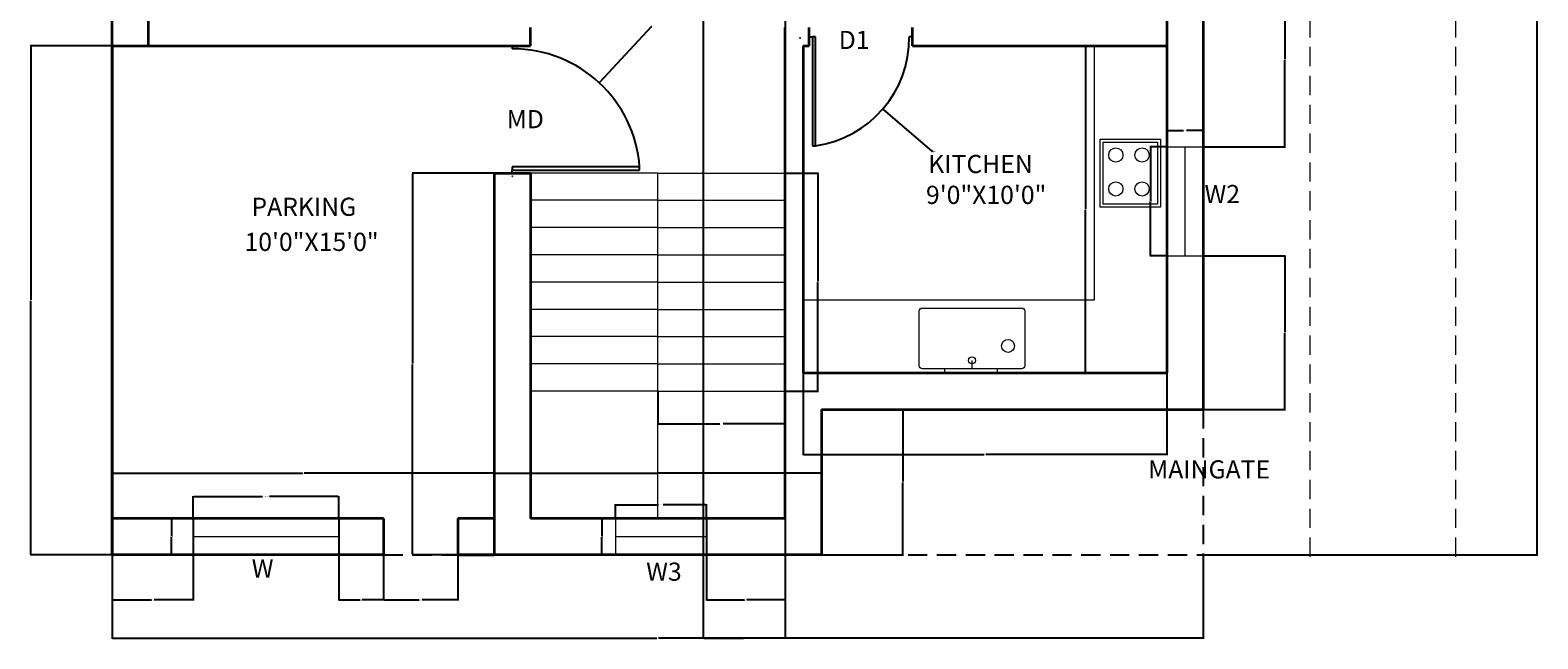
# Model space of a CAD drawing. Units: inches. Extents: x 2906 to 3403, y 1614 to 2150.
# Tile 1 of 4: x 2906 to 3403, y 1614 to 1814. Entities that reach past the tile are written whole.
import ezdxf

# ---------------------------------------------------------------- set-up
doc = ezdxf.new("R2010")
doc.units = ezdxf.units.IN
doc.linetypes.add('DASHED2', pattern=[9.525, 6.35, -3.175])
for name, color, linetype, lineweight in [('A-ANNO-DIMS', 2, 'Continuous', 18), ('A-ANNO-TEXT', 220, 'Continuous', 18), ('A-AREA-IDEN', 220, 'Continuous', 25), ('A-DOOR', 40, 'Continuous', 25), ('A-EQPM', 121, 'Continuous', 18), ('A-FLOR-CASE', 121, 'Continuous', 18), ('A-FLOR-FIXT', 121, 'Continuous', 18), ('A-FLOR-STRS', 191, 'Continuous', 18), ('A-GLAZ', 2, 'Continuous', 18), ('A-WALL', 191, 'Continuous', 35), ('C-PROP', 255, 'DASHED2', 25), ('C-ROAD', 255, 'DASHED2', 18)]:
    doc.layers.add(name, color=color, linetype=linetype, lineweight=lineweight)
doc.styles.get("Standard").update_dxf_attribs({"font": 'arial.ttf'})
doc.dimstyles.get("Standard").update_dxf_attribs({"dimtxt": 0.18, "dimasz": 0.18, "dimexe": 0.18, "dimexo": 0.0625, "dimgap": 0.09, "dimtad": 0, "dimtih": 1, "dimtoh": 1, "dimdec": 4, "dimzin": 0, "dimdsep": 46, "dimtxsty": 'Standard', "dimcen": 0.09, "dimadec": 0, "dimazin": 0, "dimtfac": 1, "dimtdec": 4, "dimtofl": 0, "dimtmove": 0, "dimatfit": 3, "dimfxl": 1, "dimtolj": 1, "dimtzin": 0, "dimarcsym": 0})

# ---------------------------------------------------------------- blocks, each defined once
blk = doc.blocks.new('WINDOW-48')
for p, q in [((0, 12), (0, 0)), ((48, 12), (48, 0)), ((0, 6), (48, 6))]:
    blk.add_line(p, q)
blk = doc.blocks.new('WINDOW-36')
for p, q in [((12, 36), (0, 36)), ((6, 36), (6, 0)), ((12, 0), (0, 0))]:
    blk.add_line(p, q)
blk = doc.blocks.new('WINDOW-30')
for p, q in [((0, 12), (0, 0)), ((30, 12), (30, 0)), ((0, 6), (30, 6))]:
    blk.add_line(p, q)
blk = doc.blocks.new('STAIR-FLIGHT-42')
for p, q in [((0, 72), (42, 72)), ((0, 63), (42, 63)), ((0, 54), (42, 54)), ((0, 45), (42, 45)), ((0, 36), (42, 36)), ((0, 27), (42, 27)), ((0, 18), (42, 18)), ((0, 9), (42, 9)), ((0, 0), (42, 0))]:
    blk.add_line(p, q)
blk = doc.blocks.new('*D18')
at = {"layer": 'A-ANNO-DIMS', "color": 0, "lineweight": -2, "transparency": 16777216}
for p, q in [((2959.37, 1653.32), (2959.37, 1660.63)), ((2959.55, 1660.45), (2982.25, 1660.45)), ((3007.19, 1660.45), (2984.49, 1660.45)), ((3007.37, 1653.32), (3007.37, 1660.63))]:
    blk.add_line(p, q, dxfattribs=at)
at = {"layer": 'A-ANNO-DIMS', "color": 0, "transparency": 16777216}
for points in [[(2959.55, 1660.48), (2959.55, 1660.42), (2959.37, 1660.45)], [(3007.19, 1660.48), (3007.19, 1660.42), (3007.37, 1660.45)]]:
    blk.add_solid(points, dxfattribs=at)
at = {"layer": 'Defpoints', "color": 0, "transparency": 16777216}
for p in [(3007.37, 1660.45), (2959.37, 1653.25), (3007.37, 1653.25)]:
    blk.add_point(p, dxfattribs=at)
at = {"layer": 'A-ANNO-DIMS', "color": 0, "transparency": 16777216, "insert": (2983.37, 1660.45), "char_height": 0.18, "attachment_point": 5}
blk.add_mtext('\\A1;WINDOW 48 TYP.', dxfattribs=at)
blk = doc.blocks.new('*D19')
at = {"layer": 'A-ANNO-DIMS', "color": 0, "lineweight": -2, "transparency": 16777216}
for p, q in [((2959.31, 1653.25), (2951.99, 1653.25)), ((2952.17, 1653.07), (2952.17, 1647.43)), ((2952.17, 1641.43), (2952.17, 1647.07)), ((2959.31, 1641.25), (2951.99, 1641.25))]:
    blk.add_line(p, q, dxfattribs=at)
at = {"layer": 'A-ANNO-DIMS', "color": 0, "transparency": 16777216}
for points in [[(2952.14, 1653.07), (2952.2, 1653.07), (2952.17, 1653.25)], [(2952.14, 1641.43), (2952.2, 1641.43), (2952.17, 1641.25)]]:
    blk.add_solid(points, dxfattribs=at)
at = {"layer": 'Defpoints', "color": 0, "transparency": 16777216}
for p in [(2952.17, 1653.25), (2959.37, 1653.25), (2959.37, 1641.25)]:
    blk.add_point(p, dxfattribs=at)
at = {"layer": 'A-ANNO-DIMS', "color": 0, "transparency": 16777216, "insert": (2952.17, 1647.25), "char_height": 0.18, "attachment_point": 5}
blk.add_mtext('\\A1;12 TYP.', dxfattribs=at)
blk = doc.blocks.new('*D22')
at = {"layer": 'A-ANNO-DIMS', "color": 0, "lineweight": -2, "transparency": 16777216}
for p, q in [((3280.57, 1775.89), (3275.05, 1775.89)), ((3275.23, 1775.71), (3275.23, 1758.08)), ((3275.23, 1740.07), (3275.23, 1757.71)), ((3280.57, 1739.89), (3275.05, 1739.89))]:
    blk.add_line(p, q, dxfattribs=at)
at = {"layer": 'A-ANNO-DIMS', "color": 0, "transparency": 16777216}
for points in [[(3275.2, 1775.71), (3275.26, 1775.71), (3275.23, 1775.89)], [(3275.2, 1740.07), (3275.26, 1740.07), (3275.23, 1739.89)]]:
    blk.add_solid(points, dxfattribs=at)
at = {"layer": 'Defpoints', "color": 0, "transparency": 16777216}
for p in [(3280.63, 1775.89), (3275.23, 1739.89), (3280.63, 1739.89)]:
    blk.add_point(p, dxfattribs=at)
at = {"layer": 'A-ANNO-DIMS', "color": 0, "transparency": 16777216, "insert": (3275.23, 1757.89), "char_height": 0.18, "attachment_point": 5}
blk.add_mtext('\\A1;W2 36 TYP.', dxfattribs=at)
blk = doc.blocks.new('*D23')
at = {"layer": 'A-ANNO-DIMS', "color": 0, "lineweight": -2, "transparency": 16777216}
for p, q in [((3280.63, 1775.96), (3280.63, 1781.47)), ((3280.81, 1781.29), (3286.11, 1781.29)), ((3292.45, 1781.29), (3287.15, 1781.29)), ((3292.63, 1775.96), (3292.63, 1781.47))]:
    blk.add_line(p, q, dxfattribs=at)
at = {"layer": 'A-ANNO-DIMS', "color": 0, "transparency": 16777216}
for points in [[(3280.81, 1781.32), (3280.81, 1781.26), (3280.63, 1781.29)], [(3292.45, 1781.32), (3292.45, 1781.26), (3292.63, 1781.29)]]:
    blk.add_solid(points, dxfattribs=at)
at = {"layer": 'Defpoints', "color": 0, "transparency": 16777216}
for p in [(3280.63, 1781.29), (3280.63, 1775.89), (3292.63, 1775.89)]:
    blk.add_point(p, dxfattribs=at)
at = {"layer": 'A-ANNO-DIMS', "color": 0, "transparency": 16777216, "insert": (3286.63, 1781.29), "char_height": 0.18, "attachment_point": 5}
blk.add_mtext('\\A1;12 TYP.', dxfattribs=at)
blk = doc.blocks.new('*D24')
at = {"layer": 'A-ANNO-DIMS', "color": 0, "lineweight": -2, "transparency": 16777216}
for p, q in [((3098.66, 1653.32), (3098.66, 1657.93)), ((3098.84, 1657.75), (3112.91, 1657.75)), ((3128.48, 1657.75), (3114.42, 1657.75)), ((3128.66, 1653.32), (3128.66, 1657.93))]:
    blk.add_line(p, q, dxfattribs=at)
at = {"layer": 'A-ANNO-DIMS', "color": 0, "transparency": 16777216}
for points in [[(3098.84, 1657.78), (3098.84, 1657.72), (3098.66, 1657.75)], [(3128.48, 1657.78), (3128.48, 1657.72), (3128.66, 1657.75)]]:
    blk.add_solid(points, dxfattribs=at)
at = {"layer": 'Defpoints', "color": 0, "transparency": 16777216}
for p in [(3128.66, 1657.75), (3098.66, 1653.25), (3128.66, 1653.25)]:
    blk.add_point(p, dxfattribs=at)
at = {"layer": 'A-ANNO-DIMS', "color": 0, "transparency": 16777216, "insert": (3113.66, 1657.75), "char_height": 0.18, "attachment_point": 5}
blk.add_mtext('\\A1;W3 30 TYP.', dxfattribs=at)
blk = doc.blocks.new('*D25')
at = {"layer": 'A-ANNO-DIMS', "color": 0, "lineweight": -2, "transparency": 16777216}
for p, q in [((3098.6, 1653.25), (3093.98, 1653.25)), ((3094.16, 1653.07), (3094.16, 1647.43)), ((3094.16, 1641.43), (3094.16, 1647.07)), ((3098.6, 1641.25), (3093.98, 1641.25))]:
    blk.add_line(p, q, dxfattribs=at)
at = {"layer": 'A-ANNO-DIMS', "color": 0, "transparency": 16777216}
for points in [[(3094.13, 1653.07), (3094.19, 1653.07), (3094.16, 1653.25)], [(3094.13, 1641.43), (3094.19, 1641.43), (3094.16, 1641.25)]]:
    blk.add_solid(points, dxfattribs=at)
at = {"layer": 'Defpoints', "color": 0, "transparency": 16777216}
for p in [(3094.16, 1653.25), (3098.66, 1653.25), (3098.66, 1641.25)]:
    blk.add_point(p, dxfattribs=at)
at = {"layer": 'A-ANNO-DIMS', "color": 0, "transparency": 16777216, "insert": (3094.16, 1647.25), "char_height": 0.18, "attachment_point": 5}
blk.add_mtext('\\A1;12 TYP.', dxfattribs=at)
blk = doc.blocks.new('*D32')
at = {"layer": 'A-ANNO-DIMS', "color": 0, "lineweight": -2, "transparency": 16777216}
for p, q in [((3154.7, 1767.25), (3165.61, 1767.25)), ((3165.43, 1767.07), (3165.43, 1731.44)), ((3165.43, 1695.43), (3165.43, 1731.07)), ((3154.7, 1695.25), (3165.61, 1695.25))]:
    blk.add_line(p, q, dxfattribs=at)
at = {"layer": 'A-ANNO-DIMS', "color": 0, "transparency": 16777216}
for points in [[(3165.4, 1767.07), (3165.46, 1767.07), (3165.43, 1767.25)], [(3165.4, 1695.43), (3165.46, 1695.43), (3165.43, 1695.25)]]:
    blk.add_solid(points, dxfattribs=at)
at = {"layer": 'Defpoints', "color": 0, "transparency": 16777216}
for p in [(3154.63, 1767.25), (3165.43, 1767.25), (3154.63, 1695.25)]:
    blk.add_point(p, dxfattribs=at)
at = {"layer": 'A-ANNO-DIMS', "color": 0, "transparency": 16777216, "insert": (3165.43, 1731.25), "char_height": 0.18, "attachment_point": 5}
blk.add_mtext('\\A1;FLIGHT 72 TYP.', dxfattribs=at)
blk = doc.blocks.new('*D33')
at = {"layer": 'A-ANNO-DIMS', "color": 0, "lineweight": -2, "transparency": 16777216}
for p, q in [((3112.63, 1695.19), (3112.63, 1684.27)), ((3154.63, 1695.19), (3154.63, 1684.27)), ((3112.81, 1684.45), (3133.1, 1684.45)), ((3154.45, 1684.45), (3134.16, 1684.45))]:
    blk.add_line(p, q, dxfattribs=at)
at = {"layer": 'A-ANNO-DIMS', "color": 0, "transparency": 16777216}
for points in [[(3112.81, 1684.48), (3112.81, 1684.42), (3112.63, 1684.45)], [(3154.45, 1684.48), (3154.45, 1684.42), (3154.63, 1684.45)]]:
    blk.add_solid(points, dxfattribs=at)
at = {"layer": 'Defpoints', "color": 0, "transparency": 16777216}
for p in [(3112.63, 1695.25), (3154.63, 1695.25), (3154.63, 1684.45)]:
    blk.add_point(p, dxfattribs=at)
at = {"layer": 'A-ANNO-DIMS', "color": 0, "transparency": 16777216, "insert": (3133.63, 1684.45), "char_height": 0.18, "attachment_point": 5}
blk.add_mtext('\\A1;42 TYP.', dxfattribs=at)
blk = doc.blocks.new('*D40')
at = {"layer": 'A-ANNO-DIMS', "color": 0, "lineweight": -2, "transparency": 16777216}
for p, q in [((2932.63, 1641.19), (2932.63, 1613.51)), ((3292.63, 1641.19), (3292.63, 1613.51)), ((2932.81, 1613.69), (3112.34, 1613.69)), ((3292.45, 1613.69), (3112.92, 1613.69))]:
    blk.add_line(p, q, dxfattribs=at)
at = {"layer": 'A-ANNO-DIMS', "color": 0, "transparency": 16777216}
for points in [[(2932.81, 1613.72), (2932.81, 1613.66), (2932.63, 1613.69)], [(3292.45, 1613.72), (3292.45, 1613.66), (3292.63, 1613.69)]]:
    blk.add_solid(points, dxfattribs=at)
at = {"layer": 'Defpoints', "color": 0, "transparency": 16777216}
for p in [(2932.63, 1641.25), (3292.63, 1641.25), (3292.63, 1613.69)]:
    blk.add_point(p, dxfattribs=at)
at = {"layer": 'A-ANNO-DIMS', "color": 0, "transparency": 16777216, "insert": (3112.63, 1613.69), "char_height": 0.18, "attachment_point": 5}
blk.add_mtext('\\A1;360', dxfattribs=at)
blk = doc.blocks.new('*D41')
at = {"layer": 'A-ANNO-DIMS', "color": 0, "lineweight": -2, "transparency": 16777216}
for p, q in [((3292.7, 2121.25), (3403.01, 2121.25)), ((3402.83, 2121.07), (3402.83, 1881.44)), ((3402.83, 1641.43), (3402.83, 1881.07)), ((3292.7, 1641.25), (3403.01, 1641.25))]:
    blk.add_line(p, q, dxfattribs=at)
at = {"layer": 'A-ANNO-DIMS', "color": 0, "transparency": 16777216}
for points in [[(3402.8, 2121.07), (3402.86, 2121.07), (3402.83, 2121.25)], [(3402.8, 1641.43), (3402.86, 1641.43), (3402.83, 1641.25)]]:
    blk.add_solid(points, dxfattribs=at)
at = {"layer": 'Defpoints', "color": 0, "transparency": 16777216}
for p in [(3292.63, 2121.25), (3402.83, 2121.25), (3292.63, 1641.25)]:
    blk.add_point(p, dxfattribs=at)
at = {"layer": 'A-ANNO-DIMS', "color": 0, "transparency": 16777216, "insert": (3402.83, 1881.25), "char_height": 0.18, "attachment_point": 5}
blk.add_mtext('\\A1;480', dxfattribs=at)
blk = doc.blocks.new('*D48')
at = {"layer": 'A-ANNO-DIMS', "color": 0, "lineweight": -2, "transparency": 16777216}
for p, q in [((2932.57, 1809.25), (2905.55, 1809.25)), ((2905.73, 1809.07), (2905.73, 1725.44)), ((2905.73, 1641.43), (2905.73, 1725.07)), ((2932.57, 1641.25), (2905.55, 1641.25))]:
    blk.add_line(p, q, dxfattribs=at)
at = {"layer": 'A-ANNO-DIMS', "color": 0, "transparency": 16777216}
for points in [[(2905.7, 1809.07), (2905.76, 1809.07), (2905.73, 1809.25)], [(2905.7, 1641.43), (2905.76, 1641.43), (2905.73, 1641.25)]]:
    blk.add_solid(points, dxfattribs=at)
at = {"layer": 'Defpoints', "color": 0, "transparency": 16777216}
for p in [(2905.73, 1809.25), (2932.63, 1809.25), (2932.63, 1641.25)]:
    blk.add_point(p, dxfattribs=at)
at = {"layer": 'A-ANNO-DIMS', "color": 0, "transparency": 16777216, "insert": (2905.73, 1725.25), "char_height": 0.18, "attachment_point": 5}
blk.add_mtext('\\A1;168', dxfattribs=at)
blk = doc.blocks.new('*D52')
at = {"layer": 'A-ANNO-DIMS', "color": 0, "lineweight": -2, "transparency": 16777216}
for p, q in [((2932.63, 1641.32), (2932.63, 1668.33)), ((2932.81, 1668.15), (2995.35, 1668.15)), ((3058.45, 1668.15), (2995.91, 1668.15)), ((3058.63, 1641.32), (3058.63, 1668.33))]:
    blk.add_line(p, q, dxfattribs=at)
at = {"layer": 'A-ANNO-DIMS', "color": 0, "transparency": 16777216}
for points in [[(2932.81, 1668.18), (2932.81, 1668.12), (2932.63, 1668.15)], [(3058.45, 1668.18), (3058.45, 1668.12), (3058.63, 1668.15)]]:
    blk.add_solid(points, dxfattribs=at)
at = {"layer": 'Defpoints', "color": 0, "transparency": 16777216}
for p in [(3058.63, 1668.15), (2932.63, 1641.25), (3058.63, 1641.25)]:
    blk.add_point(p, dxfattribs=at)
at = {"layer": 'A-ANNO-DIMS', "color": 0, "transparency": 16777216, "insert": (2995.63, 1668.15), "char_height": 0.18, "attachment_point": 5}
blk.add_mtext('\\A1;126', dxfattribs=at)
blk = doc.blocks.new('*D53')
at = {"layer": 'A-ANNO-DIMS', "color": 0, "lineweight": -2, "transparency": 16777216}
for p, q in [((3058.63, 1641.32), (3058.63, 1668.33)), ((3058.81, 1668.15), (3112.35, 1668.15)), ((3166.45, 1668.15), (3112.91, 1668.15)), ((3166.63, 1641.32), (3166.63, 1668.33))]:
    blk.add_line(p, q, dxfattribs=at)
at = {"layer": 'A-ANNO-DIMS', "color": 0, "transparency": 16777216}
for points in [[(3058.81, 1668.18), (3058.81, 1668.12), (3058.63, 1668.15)], [(3166.45, 1668.18), (3166.45, 1668.12), (3166.63, 1668.15)]]:
    blk.add_solid(points, dxfattribs=at)
at = {"layer": 'Defpoints', "color": 0, "transparency": 16777216}
for p in [(3166.63, 1668.15), (3058.63, 1641.25), (3166.63, 1641.25)]:
    blk.add_point(p, dxfattribs=at)
at = {"layer": 'A-ANNO-DIMS', "color": 0, "transparency": 16777216, "insert": (3112.63, 1668.15), "char_height": 0.18, "attachment_point": 5}
blk.add_mtext('\\A1;108', dxfattribs=at)
blk = doc.blocks.new('*D54')
at = {"layer": 'A-ANNO-DIMS', "color": 0, "lineweight": -2, "transparency": 16777216}
for p, q in [((2932.63, 1653.19), (2932.63, 1626.17)), ((2959.37, 1653.19), (2959.37, 1626.17)), ((2932.81, 1626.35), (2945.53, 1626.35)), ((2959.19, 1626.35), (2946.47, 1626.35))]:
    blk.add_line(p, q, dxfattribs=at)
at = {"layer": 'A-ANNO-DIMS', "color": 0, "transparency": 16777216}
for points in [[(2932.81, 1626.38), (2932.81, 1626.32), (2932.63, 1626.35)], [(2959.19, 1626.38), (2959.19, 1626.32), (2959.37, 1626.35)]]:
    blk.add_solid(points, dxfattribs=at)
at = {"layer": 'Defpoints', "color": 0, "transparency": 16777216}
for p in [(2932.63, 1653.25), (2959.37, 1653.25), (2932.63, 1626.35)]:
    blk.add_point(p, dxfattribs=at)
at = {"layer": 'A-ANNO-DIMS', "color": 0, "transparency": 16777216, "insert": (2946, 1626.35), "char_height": 0.18, "attachment_point": 5}
blk.add_mtext('\\A1;26.735', dxfattribs=at)
blk = doc.blocks.new('*D55')
at = {"layer": 'A-ANNO-DIMS', "color": 0, "lineweight": -2, "transparency": 16777216}
for p, q in [((3007.37, 1653.19), (3007.37, 1626.17)), ((3022.17, 1653.19), (3022.17, 1626.17)), ((3007.55, 1626.35), (3014.45, 1626.35)), ((3021.99, 1626.35), (3015.08, 1626.35))]:
    blk.add_line(p, q, dxfattribs=at)
at = {"layer": 'A-ANNO-DIMS', "color": 0, "transparency": 16777216}
for points in [[(3007.55, 1626.38), (3007.55, 1626.32), (3007.37, 1626.35)], [(3021.99, 1626.38), (3021.99, 1626.32), (3022.17, 1626.35)]]:
    blk.add_solid(points, dxfattribs=at)
at = {"layer": 'Defpoints', "color": 0, "transparency": 16777216}
for p in [(3007.37, 1653.25), (3022.17, 1653.25), (3007.37, 1626.35)]:
    blk.add_point(p, dxfattribs=at)
at = {"layer": 'A-ANNO-DIMS', "color": 0, "transparency": 16777216, "insert": (3014.77, 1626.35), "char_height": 0.18, "attachment_point": 5}
blk.add_mtext('\\A1;14.8', dxfattribs=at)
blk = doc.blocks.new('*D56')
at = {"layer": 'A-ANNO-DIMS', "color": 0, "lineweight": -2, "transparency": 16777216}
for p, q in [((3022.17, 1653.19), (3022.17, 1626.17)), ((3046.63, 1653.19), (3046.63, 1626.17)), ((3022.35, 1626.35), (3033.93, 1626.35)), ((3046.45, 1626.35), (3034.86, 1626.35))]:
    blk.add_line(p, q, dxfattribs=at)
at = {"layer": 'A-ANNO-DIMS', "color": 0, "transparency": 16777216}
for points in [[(3022.35, 1626.38), (3022.35, 1626.32), (3022.17, 1626.35)], [(3046.45, 1626.38), (3046.45, 1626.32), (3046.63, 1626.35)]]:
    blk.add_solid(points, dxfattribs=at)
at = {"layer": 'Defpoints', "color": 0, "transparency": 16777216}
for p in [(3022.17, 1653.25), (3046.63, 1653.25), (3022.17, 1626.35)]:
    blk.add_point(p, dxfattribs=at)
at = {"layer": 'A-ANNO-DIMS', "color": 0, "transparency": 16777216, "insert": (3034.4, 1626.35), "char_height": 0.18, "attachment_point": 5}
blk.add_mtext('\\A1;24.466', dxfattribs=at)
blk = doc.blocks.new('*D57')
at = {"layer": 'A-ANNO-DIMS', "color": 0, "lineweight": -2, "transparency": 16777216}
for p, q in [((3128.66, 1653.19), (3128.66, 1626.17)), ((3154.63, 1653.19), (3154.63, 1626.17)), ((3128.84, 1626.35), (3141.25, 1626.35)), ((3154.45, 1626.35), (3142.04, 1626.35))]:
    blk.add_line(p, q, dxfattribs=at)
at = {"layer": 'A-ANNO-DIMS', "color": 0, "transparency": 16777216}
for points in [[(3128.84, 1626.38), (3128.84, 1626.32), (3128.66, 1626.35)], [(3154.45, 1626.38), (3154.45, 1626.32), (3154.63, 1626.35)]]:
    blk.add_solid(points, dxfattribs=at)
at = {"layer": 'Defpoints', "color": 0, "transparency": 16777216}
for p in [(3128.66, 1653.25), (3154.63, 1653.25), (3128.66, 1626.35)]:
    blk.add_point(p, dxfattribs=at)
at = {"layer": 'A-ANNO-DIMS', "color": 0, "transparency": 16777216, "insert": (3141.65, 1626.35), "char_height": 0.18, "attachment_point": 5}
blk.add_mtext('\\A1;25.97', dxfattribs=at)
blk = doc.blocks.new('*D58')
at = {"layer": 'A-ANNO-DIMS', "color": 0, "lineweight": -2, "transparency": 16777216}
for p, q in [((3058.57, 1767.25), (3031.55, 1767.25)), ((3031.73, 1767.07), (3031.73, 1704.44)), ((3031.73, 1641.43), (3031.73, 1704.07)), ((3058.57, 1641.25), (3031.55, 1641.25))]:
    blk.add_line(p, q, dxfattribs=at)
at = {"layer": 'A-ANNO-DIMS', "color": 0, "transparency": 16777216}
for points in [[(3031.7, 1767.07), (3031.76, 1767.07), (3031.73, 1767.25)], [(3031.7, 1641.43), (3031.76, 1641.43), (3031.73, 1641.25)]]:
    blk.add_solid(points, dxfattribs=at)
at = {"layer": 'Defpoints', "color": 0, "transparency": 16777216}
for p in [(3031.73, 1767.25), (3058.63, 1767.25), (3058.63, 1641.25)]:
    blk.add_point(p, dxfattribs=at)
at = {"layer": 'A-ANNO-DIMS', "color": 0, "transparency": 16777216, "insert": (3031.73, 1704.25), "char_height": 0.18, "attachment_point": 5}
blk.add_mtext('\\A1;126', dxfattribs=at)
blk = doc.blocks.new('*D60')
at = {"layer": 'A-ANNO-DIMS', "color": 0, "lineweight": -2, "transparency": 16777216}
for p, q in [((3160.63, 1701.19), (3160.63, 1674.17)), ((3280.63, 1701.19), (3280.63, 1674.17)), ((3160.81, 1674.35), (3220.35, 1674.35)), ((3280.45, 1674.35), (3220.91, 1674.35))]:
    blk.add_line(p, q, dxfattribs=at)
at = {"layer": 'A-ANNO-DIMS', "color": 0, "transparency": 16777216}
for points in [[(3160.81, 1674.38), (3160.81, 1674.32), (3160.63, 1674.35)], [(3280.45, 1674.38), (3280.45, 1674.32), (3280.63, 1674.35)]]:
    blk.add_solid(points, dxfattribs=at)
at = {"layer": 'Defpoints', "color": 0, "transparency": 16777216}
for p in [(3160.63, 1701.25), (3280.63, 1701.25), (3160.63, 1674.35)]:
    blk.add_point(p, dxfattribs=at)
at = {"layer": 'A-ANNO-DIMS', "color": 0, "transparency": 16777216, "insert": (3220.63, 1674.35), "char_height": 0.18, "attachment_point": 5}
blk.add_mtext('\\A1;120', dxfattribs=at)
blk = doc.blocks.new('*D61')
at = {"layer": 'A-ANNO-DIMS', "color": 0, "lineweight": -2, "transparency": 16777216}
for p, q in [((3280.57, 1809.25), (3253.55, 1809.25)), ((3253.73, 1809.07), (3253.73, 1755.44)), ((3253.73, 1701.43), (3253.73, 1755.07)), ((3280.57, 1701.25), (3253.55, 1701.25))]:
    blk.add_line(p, q, dxfattribs=at)
at = {"layer": 'A-ANNO-DIMS', "color": 0, "transparency": 16777216}
for points in [[(3253.7, 1809.07), (3253.76, 1809.07), (3253.73, 1809.25)], [(3253.7, 1701.43), (3253.76, 1701.43), (3253.73, 1701.25)]]:
    blk.add_solid(points, dxfattribs=at)
at = {"layer": 'Defpoints', "color": 0, "transparency": 16777216}
for p in [(3253.73, 1809.25), (3280.63, 1809.25), (3280.63, 1701.25)]:
    blk.add_point(p, dxfattribs=at)
at = {"layer": 'A-ANNO-DIMS', "color": 0, "transparency": 16777216, "insert": (3253.73, 1755.25), "char_height": 0.18, "attachment_point": 5}
blk.add_mtext('\\A1;108', dxfattribs=at)
blk = doc.blocks.new('*D64')
at = {"layer": 'A-ANNO-DIMS', "color": 0, "lineweight": -2, "transparency": 16777216}
for p, q in [((3166.7, 1689.25), (3193.71, 1689.25)), ((3193.53, 1689.07), (3193.53, 1665.44)), ((3193.53, 1641.43), (3193.53, 1665.07)), ((3166.7, 1641.25), (3193.71, 1641.25))]:
    blk.add_line(p, q, dxfattribs=at)
at = {"layer": 'A-ANNO-DIMS', "color": 0, "transparency": 16777216}
for points in [[(3193.5, 1689.07), (3193.56, 1689.07), (3193.53, 1689.25)], [(3193.5, 1641.43), (3193.56, 1641.43), (3193.53, 1641.25)]]:
    blk.add_solid(points, dxfattribs=at)
at = {"layer": 'Defpoints', "color": 0, "transparency": 16777216}
for p in [(3166.63, 1689.25), (3166.63, 1641.25), (3193.53, 1641.25)]:
    blk.add_point(p, dxfattribs=at)
at = {"layer": 'A-ANNO-DIMS', "color": 0, "transparency": 16777216, "insert": (3193.53, 1665.25), "char_height": 0.18, "attachment_point": 5}
blk.add_mtext('\\A1;48', dxfattribs=at)
blk = doc.blocks.new('*D69')
at = {"layer": 'A-ANNO-DIMS', "color": 0, "lineweight": -2, "transparency": 16777216}
for p, q in [((3292.7, 1833.53), (3319.71, 1833.53)), ((3319.53, 1833.35), (3319.53, 1804.89)), ((3319.53, 1776.07), (3319.53, 1804.53)), ((3292.7, 1775.89), (3319.71, 1775.89))]:
    blk.add_line(p, q, dxfattribs=at)
at = {"layer": 'A-ANNO-DIMS', "color": 0, "transparency": 16777216}
for points in [[(3319.5, 1833.35), (3319.56, 1833.35), (3319.53, 1833.53)], [(3319.5, 1776.07), (3319.56, 1776.07), (3319.53, 1775.89)]]:
    blk.add_solid(points, dxfattribs=at)
at = {"layer": 'Defpoints', "color": 0, "transparency": 16777216}
for p in [(3292.63, 1833.53), (3292.63, 1775.89), (3319.53, 1775.89)]:
    blk.add_point(p, dxfattribs=at)
at = {"layer": 'A-ANNO-DIMS', "color": 0, "transparency": 16777216, "insert": (3319.53, 1804.71), "char_height": 0.18, "attachment_point": 5}
blk.add_mtext('\\A1;57.63', dxfattribs=at)
blk = doc.blocks.new('*D70')
at = {"layer": 'A-ANNO-DIMS', "color": 0, "lineweight": -2, "transparency": 16777216}
for p, q in [((3292.7, 1739.89), (3319.71, 1739.89)), ((3319.53, 1739.71), (3319.53, 1714.76)), ((3319.53, 1689.43), (3319.53, 1714.39)), ((3292.7, 1689.25), (3319.71, 1689.25))]:
    blk.add_line(p, q, dxfattribs=at)
at = {"layer": 'A-ANNO-DIMS', "color": 0, "transparency": 16777216}
for points in [[(3319.5, 1739.71), (3319.56, 1739.71), (3319.53, 1739.89)], [(3319.5, 1689.43), (3319.56, 1689.43), (3319.53, 1689.25)]]:
    blk.add_solid(points, dxfattribs=at)
at = {"layer": 'Defpoints', "color": 0, "transparency": 16777216}
for p in [(3292.63, 1739.89), (3292.63, 1689.25), (3319.53, 1689.25)]:
    blk.add_point(p, dxfattribs=at)
at = {"layer": 'A-ANNO-DIMS', "color": 0, "transparency": 16777216, "insert": (3319.53, 1714.57), "char_height": 0.18, "attachment_point": 5}
blk.add_mtext('\\A1;50.64', dxfattribs=at)
blk = doc.blocks.new('*D75')
at = {"layer": 'A-ANNO-DIMS', "color": 0, "lineweight": -2, "transparency": 16777216}
for p, q in [((3127.63, 2013.19), (3127.63, 1613.51)), ((3154.63, 2013.19), (3154.63, 1613.51)), ((3127.81, 1613.69), (3140.91, 1613.69)), ((3154.45, 1613.69), (3141.35, 1613.69))]:
    blk.add_line(p, q, dxfattribs=at)
at = {"layer": 'A-ANNO-DIMS', "color": 0, "transparency": 16777216}
for points in [[(3127.81, 1613.72), (3127.81, 1613.66), (3127.63, 1613.69)], [(3154.45, 1613.72), (3154.45, 1613.66), (3154.63, 1613.69)]]:
    blk.add_solid(points, dxfattribs=at)
at = {"layer": 'Defpoints', "color": 0, "transparency": 16777216}
for p in [(3127.63, 2013.25), (3154.63, 2013.25), (3154.63, 1613.69)]:
    blk.add_point(p, dxfattribs=at)
at = {"layer": 'A-ANNO-DIMS', "color": 0, "transparency": 16777216, "insert": (3141.13, 1613.69), "char_height": 0.18, "attachment_point": 5}
blk.add_mtext('\\A1;27', dxfattribs=at)
blk = doc.blocks.new('*D80')
at = {"layer": 'A-ANNO-DIMS', "color": 0, "lineweight": -2, "transparency": 16777216}
for p, q in [((3110.47, 1815.5), (3093.44, 1797.16)), ((3110.65, 1815.5), (3110.47, 1815.5)), ((3064.65, 1766.25), (3064.83, 1766.25)), ((3064.74, 1766.16), (3064.74, 1766.34))]:
    blk.add_line(p, q, dxfattribs=at)
at = {"layer": 'A-ANNO-DIMS', "color": 0, "transparency": 16777216}
blk.add_solid([(3093.42, 1797.18), (3093.46, 1797.14), (3093.32, 1797.03)], dxfattribs=at)
at = {"layer": 'Defpoints', "color": 0, "transparency": 16777216}
for p in [(3093.32, 1797.03), (3064.74, 1766.25)]:
    blk.add_point(p, dxfattribs=at)
at = {"layer": 'A-ANNO-DIMS', "color": 0, "transparency": 16777216, "insert": (3110.95, 1815.5), "char_height": 0.18, "attachment_point": 5}
blk.add_mtext('\\A1;R42', dxfattribs=at)
blk = doc.blocks.new('*D81')
at = {"layer": 'A-ANNO-DIMS', "color": 0, "lineweight": -2, "transparency": 16777216}
for p, q in [((3159.54, 1811.91), (3159.72, 1811.91)), ((3159.63, 1811.82), (3159.63, 1812)), ((3203.28, 1774.32), (3187.05, 1788.3)), ((3203.46, 1774.32), (3203.28, 1774.32))]:
    blk.add_line(p, q, dxfattribs=at)
at = {"layer": 'A-ANNO-DIMS', "color": 0, "transparency": 16777216}
blk.add_solid([(3187.07, 1788.32), (3187.03, 1788.27), (3186.91, 1788.41)], dxfattribs=at)
at = {"layer": 'Defpoints', "color": 0, "transparency": 16777216}
for p in [(3159.63, 1811.91), (3186.91, 1788.41)]:
    blk.add_point(p, dxfattribs=at)
at = {"layer": 'A-ANNO-DIMS', "color": 0, "transparency": 16777216, "insert": (3203.96, 1774.32), "char_height": 0.18, "attachment_point": 5}
blk.add_mtext('\\A1;3X R36', dxfattribs=at)

msp = doc.modelspace()

# ---------------------------------------------------------------- linework, layer by layer
at = {"layer": 'A-DOOR'}
for p, q in [((3162.6325, 1812.254), (3163.6325, 1812.254)), ((3163.6325, 1812.254), (3163.6325, 1776.254)), ((3164.6325, 1812.254), (3163.6325, 1812.254)), ((3164.6325, 1776.254), (3164.6325, 1812.254)), ((3196.6325, 1812.254), (3195.6325, 1812.254)), ((3064.6325, 1809.254), (3064.6325, 1808.254)), ((3163.6325, 1776.254), (3164.6325, 1776.254)), ((3106.6325, 1769.254), (3064.6325, 1769.254)), ((3064.6325, 1769.254), (3064.6325, 1768.254)), ((3064.6325, 1767.254), (3064.6325, 1768.254)), ((3064.6325, 1768.254), (3106.6325, 1768.254)), ((3106.6325, 1768.254), (3106.6325, 1769.254))]:
    msp.add_line(p, q, dxfattribs=at)
for centre, radius, start, end in [((3159.6342, 1811.9053), 36, 277.980842, 0.554944), ((3064.7398, 1766.2541), 42, 4.095856, 90.146336)]:
    msp.add_arc(centre, radius, start, end, dxfattribs=at)
at = {"layer": 'A-EQPM'}
for points in [[(3258.5931, 1778.4157), (3278.5455, 1778.4157), (3278.5455, 1755.9711), (3258.5931, 1755.9711)], [(3259.5931, 1777.4157), (3277.5455, 1777.4157), (3277.5455, 1756.9711), (3259.5931, 1756.9711)]]:
    msp.add_lwpolyline(points, close=True, dxfattribs=at)
for centre in [(3263.7787, 1773.1937), (3272.4406, 1773.1937), (3263.7787, 1762.0042), (3272.4406, 1762.0042)]:
    msp.add_circle(centre, 2.354, dxfattribs=at)
at = {"layer": 'A-FLOR-CASE'}
for p, q in [((3280.6325, 1809.254), (3256.6325, 1809.254)), ((3256.6325, 1809.254), (3256.6325, 1725.254)), ((3256.6325, 1725.254), (3160.6325, 1725.254))]:
    msp.add_line(p, q, dxfattribs=at)
at = {"layer": 'A-FLOR-FIXT'}
for p, q in [((3207.2013, 1702.656), (3207.2013, 1701.254)), ((3216.3184, 1702.656), (3216.3184, 1705.4241)), ((3224.7004, 1701.254), (3224.7004, 1702.656)), ((3207.2013, 1701.254), (3224.7004, 1701.254))]:
    msp.add_line(p, q, dxfattribs=at)
msp.add_lwpolyline([(3199.8813, 1722.6985), (3232.7555, 1722.6985, -0.41421356), (3233.7555, 1721.6985), (3233.7555, 1703.656, -0.41421356), (3232.7555, 1702.656), (3199.8813, 1702.656, -0.41421356), (3198.8813, 1703.656), (3198.8813, 1721.6985, -0.41421356)], format="xyb", close=True, dxfattribs=at)
for centre, radius in [((3228.2075, 1710.2011), 2.1356), ((3216.3184, 1705.4241), 1.1802)]:
    msp.add_circle(centre, radius, dxfattribs=at)
at = {"layer": 'A-FLOR-STRS'}
msp.add_line((3112.6325, 1653.254), (3112.6325, 1767.254), dxfattribs=at)
at = {"layer": 'A-WALL'}
for p, q in [((2944.6325, 1809.254), (2944.6325, 2109.254)), ((3280.6325, 2109.254), (3280.6325, 1701.254)), ((3070.6325, 1809.254), (3070.6325, 1815.254)), ((3154.6325, 1653.254), (3154.6325, 1815.254)), ((3162.6325, 1809.254), (3162.6325, 1815.254)), ((3196.6325, 1809.254), (3196.6325, 1815.254)), ((2932.6325, 1809.254), (3070.6325, 1809.254)), ((2932.6325, 1809.254), (2932.6325, 1641.254)), ((3160.6325, 1809.254), (3162.6325, 1809.254)), ((3160.6325, 1809.254), (3160.6325, 1701.254)), ((3196.6325, 1809.254), (3280.6325, 1809.254)), ((3058.6325, 1767.254), (3058.6325, 1641.254)), ((3058.6325, 1767.254), (3070.6325, 1767.254)), ((3070.6325, 1767.254), (3070.6325, 1653.254)), ((3160.6325, 1701.254), (3166.6325, 1701.254)), ((3166.6325, 1701.254), (3280.6325, 1701.254)), ((3166.6325, 1689.254), (3292.6325, 1689.254)), ((3166.6325, 1689.254), (3166.6325, 1641.254)), ((3022.1668, 1653.254), (2932.6325, 1653.254)), ((3022.1668, 1653.254), (3022.1668, 1641.254)), ((3058.6325, 1653.254), (3046.6325, 1653.254)), ((3046.6325, 1653.254), (3046.6325, 1641.254)), ((3154.6325, 1653.254), (3070.6325, 1653.254)), ((3046.6325, 1641.254), (3058.6325, 1641.254))]:
    msp.add_line(p, q, dxfattribs=at)
for points in [[(3022.1668, 1641.254), (2932.6325, 1641.254), (2932.6325, 2121.254), (3292.6325, 2121.254), (3292.6325, 1689.254)], [(3166.6325, 1641.254), (3046.6325, 1641.254)]]:
    msp.add_lwpolyline(points, dxfattribs=at)
at = {"layer": 'C-PROP'}
for p, q in [((3292.6325, 1689.254), (3292.6325, 1641.254)), ((3022.1668, 1641.254), (3046.6325, 1641.254)), ((3166.6325, 1641.254), (3292.6325, 1641.254))]:
    msp.add_line(p, q, dxfattribs=at)
at = {"layer": 'C-ROAD'}
for p, q in [((3327.9288, 1640.586), (3327.9288, 2122.8771)), ((3375.9288, 1640.586), (3375.9288, 2122.8771))]:
    msp.add_line(p, q, dxfattribs=at)

# ---------------------------------------------------------------- block references
at = {"layer": 'A-FLOR-STRS', "rotation": 180}
msp.add_blockref('STAIR-FLIGHT-42', (3112.632, 1767.2539), dxfattribs=at)
at = {"layer": 'A-FLOR-STRS'}
msp.add_blockref('STAIR-FLIGHT-42', (3112.633, 1695.254), dxfattribs=at)
at = {"layer": 'A-GLAZ', "rotation": 180}
msp.add_blockref('WINDOW-36', (3292.632, 1775.8952), dxfattribs=at)
at = {"layer": 'A-GLAZ'}
for name, p in [('WINDOW-48', (2959.3677, 1641.254)), ('WINDOW-30', (3098.662, 1641.254))]:
    msp.add_blockref(name, p, dxfattribs=at)

# ---------------------------------------------------------------- texts
at = {"layer": 'A-ANNO-TEXT'}
for tag, p in [('D1', (3172.3268, 1808.183)), ('MD', (3062.7701, 1782.04)), ('W2', (3293.0386, 1757.3289)), ('MAINGATE', (3274.4258, 1666.4329)), ('W', (2978.6386, 1633.7031)), ('W3', (3108.8002, 1632.6839))]:
    msp.add_attdef(tag, p, '', height=6, dxfattribs=at)
at = {"layer": 'A-AREA-IDEN'}
for tag, p in [('KITCHEN', (3201.8745, 1767.2359)), ('9\'0"X10\'0"', (3201.1314, 1757.0528)), ('PARKING', (2978.5286, 1753.1179)), ('10\'0"X15\'0"', (2976.2573, 1741.5359))]:
    msp.add_attdef(tag, p, '', height=6, dxfattribs=at)

# ---------------------------------------------------------------- dimensions: what is measured, and where the dimension line sits
at = {"layer": 'A-ANNO-DIMS'}
for base, p1, p2, angle, override, picture, middle in [((3402.8288, 2121.254), (3292.6325, 1641.254), (3292.6325, 2121.254), 90, {"dimdec": 0, "dimlfac": 1, "dimrnd": 0, "dimzin": 0, "dimdsep": 46, "dimlunit": 2}, '*D41', (3402.8288, 1881.254)), ((3319.5325, 1775.8947), (3292.6325, 1833.5286), (3292.6325, 1775.8947), 270, {"dimdec": 2, "dimlfac": 1, "dimrnd": 0, "dimzin": 0, "dimdsep": 46, "dimlunit": 2}, '*D69', (3319.5325, 1804.7116)), ((2905.7325, 1809.254), (2932.6325, 1641.254), (2932.6325, 1809.254), 90, {"dimdec": 0, "dimlfac": 1, "dimrnd": 0, "dimzin": 0, "dimdsep": 46, "dimlunit": 2}, '*D48', (2905.7325, 1725.254)), ((3253.7325, 1809.254), (3280.6325, 1701.254), (3280.6325, 1809.254), 90, {"dimdec": 0, "dimlfac": 1, "dimrnd": 0, "dimzin": 0, "dimdsep": 46, "dimlunit": 2}, '*D61', (3253.7325, 1755.254)), ((3031.7325, 1767.254), (3058.6325, 1641.254), (3058.6325, 1767.254), 90, {"dimdec": 0, "dimlfac": 1, "dimrnd": 0, "dimzin": 0, "dimdsep": 46, "dimlunit": 2}, '*D58', (3031.7325, 1704.254)), ((3319.5325, 1689.254), (3292.6325, 1739.8947), (3292.6325, 1689.254), 270, {"dimdec": 2, "dimlfac": 1, "dimrnd": 0, "dimzin": 0, "dimdsep": 46, "dimlunit": 2}, '*D70', (3319.5325, 1714.5743)), ((3160.6325, 1674.354), (3280.6325, 1701.254), (3160.6325, 1701.254), 180, {"dimdec": 0, "dimlfac": 1, "dimrnd": 0, "dimzin": 0, "dimdsep": 46, "dimlunit": 2}, '*D60', (3220.6325, 1674.354)), ((3193.5325, 1641.254), (3166.6325, 1689.254), (3166.6325, 1641.254), 270, {"dimdec": 0, "dimlfac": 1, "dimrnd": 0, "dimzin": 0, "dimdsep": 46, "dimlunit": 2}, '*D64', (3193.5325, 1665.254)), ((2932.63252, 1626.35397), (2959.36801, 1653.25397), (2932.63252, 1653.25397), 180, {"dimdec": 3, "dimlfac": 1, "dimrnd": 0, "dimzin": 0, "dimdsep": 46, "dimlunit": 2}, '*D54', (2946.00027, 1626.35397)), ((3007.368, 1626.354), (3022.1668, 1653.254), (3007.368, 1653.254), 180, {"dimdec": 1, "dimlfac": 1, "dimrnd": 0, "dimzin": 0, "dimdsep": 46, "dimlunit": 2}, '*D55', (3014.7674, 1626.354)), ((3022.1668, 1626.354), (3046.6325, 1653.254), (3022.1668, 1653.254), 180, {"dimdec": 3, "dimlfac": 1, "dimrnd": 0, "dimzin": 0, "dimdsep": 46, "dimlunit": 2}, '*D56', (3034.3996, 1626.354)), ((3128.662, 1626.354), (3154.6325, 1653.254), (3128.662, 1653.254), 180, {"dimdec": 2, "dimlfac": 1, "dimrnd": 0, "dimzin": 0, "dimdsep": 46, "dimlunit": 2}, '*D57', (3141.6473, 1626.354))]:
    dim = msp.add_linear_dim(base=base, p1=p1, p2=p2, angle=angle, dimstyle='Standard', override=override, dxfattribs=at)
    dim.commit()
    dim.dimension.update_dxf_attribs({"geometry": picture, "text_midpoint": middle})
for base, p1, p2, picture, middle in [((3154.6325, 1613.686), (3127.6325, 2013.254), (3154.6325, 2013.254), '*D75', (3141.1325, 1613.686)), ((3058.6325, 1668.154), (2932.6325, 1641.254), (3058.6325, 1641.254), '*D52', (2995.6325, 1668.154)), ((3166.6325, 1668.154), (3058.6325, 1641.254), (3166.6325, 1641.254), '*D53', (3112.6325, 1668.154)), ((3292.6325, 1613.686), (2932.6325, 1641.254), (3292.6325, 1641.254), '*D40', (3112.6325, 1613.686))]:
    dim = msp.add_linear_dim(base=base, p1=p1, p2=p2, dimstyle='Standard', override={"dimdec": 0, "dimlfac": 1, "dimrnd": 0, "dimzin": 0, "dimdsep": 46, "dimlunit": 2}, dxfattribs=at)
    dim.commit()
    dim.dimension.update_dxf_attribs({"geometry": picture, "text_midpoint": middle})
dim = msp.add_radius_dim(center=(3064.7398, 1766.2541), mpoint=(3093.3191, 1797.0311), dimstyle='Standard', override={"dimdec": 0, "dimlfac": 1, "dimrnd": 0, "dimzin": 0, "dimdsep": 46, "dimlunit": 2}, dxfattribs=at)
dim.commit()
dim.dimension.update_dxf_attribs({"geometry": '*D80', "text_midpoint": (3110.9508, 1815.4973), "dimtype": 164})
dim = msp.add_radius_dim(center=(3159.6342, 1811.9053), mpoint=(3186.9137, 1788.4143), text='3X <>', dimstyle='Standard', override={"dimdec": 0, "dimlfac": 1, "dimrnd": 0, "dimzin": 0, "dimdsep": 46, "dimlunit": 2}, dxfattribs=at)
dim.commit()
dim.dimension.update_dxf_attribs({"geometry": '*D81', "text_midpoint": (3203.9597, 1774.3196), "dimtype": 164})
for base, p1, p2, angle, text, picture, middle in [((3280.6325, 1781.2947), (3292.6325, 1775.8947), (3280.6325, 1775.8947), 180, '<> TYP.', '*D23', (3286.6325, 1781.2947)), ((3275.2325, 1739.8947), (3280.6325, 1775.8947), (3280.6325, 1739.8947), 270, 'W2 <> TYP.', '*D22', (3275.2325, 1757.8947)), ((3165.4325, 1767.254), (3154.6325, 1695.254), (3154.6325, 1767.254), 90, 'FLIGHT <> TYP.', '*D32', (3165.4325, 1731.254)), ((2952.168, 1653.254), (2959.368, 1641.254), (2959.368, 1653.254), 90, '<> TYP.', '*D19', (2952.168, 1647.254)), ((3094.162, 1653.254), (3098.662, 1641.254), (3098.662, 1653.254), 90, '<> TYP.', '*D25', (3094.162, 1647.254))]:
    dim = msp.add_linear_dim(base=base, p1=p1, p2=p2, angle=angle, text=text, dimstyle='Standard', override={"dimdec": 0, "dimlfac": 1, "dimrnd": 0, "dimzin": 0, "dimdsep": 46, "dimlunit": 2}, dxfattribs=at)
    dim.commit()
    dim.dimension.update_dxf_attribs({"geometry": picture, "text_midpoint": middle})
for base, p1, p2, text, picture, middle in [((3154.6325, 1684.454), (3112.6325, 1695.254), (3154.6325, 1695.254), '<> TYP.', '*D33', (3133.6325, 1684.454)), ((3007.368, 1660.454), (2959.368, 1653.254), (3007.368, 1653.254), 'WINDOW <> TYP.', '*D18', (2983.368, 1660.454)), ((3128.662, 1657.754), (3098.662, 1653.254), (3128.662, 1653.254), 'W3 <> TYP.', '*D24', (3113.662, 1657.754))]:
    dim = msp.add_linear_dim(base=base, p1=p1, p2=p2, text=text, dimstyle='Standard', override={"dimdec": 0, "dimlfac": 1, "dimrnd": 0, "dimzin": 0, "dimdsep": 46, "dimlunit": 2}, dxfattribs=at)
    dim.commit()
    dim.dimension.update_dxf_attribs({"geometry": picture, "text_midpoint": middle})

doc.saveas('drawing.dxf')
